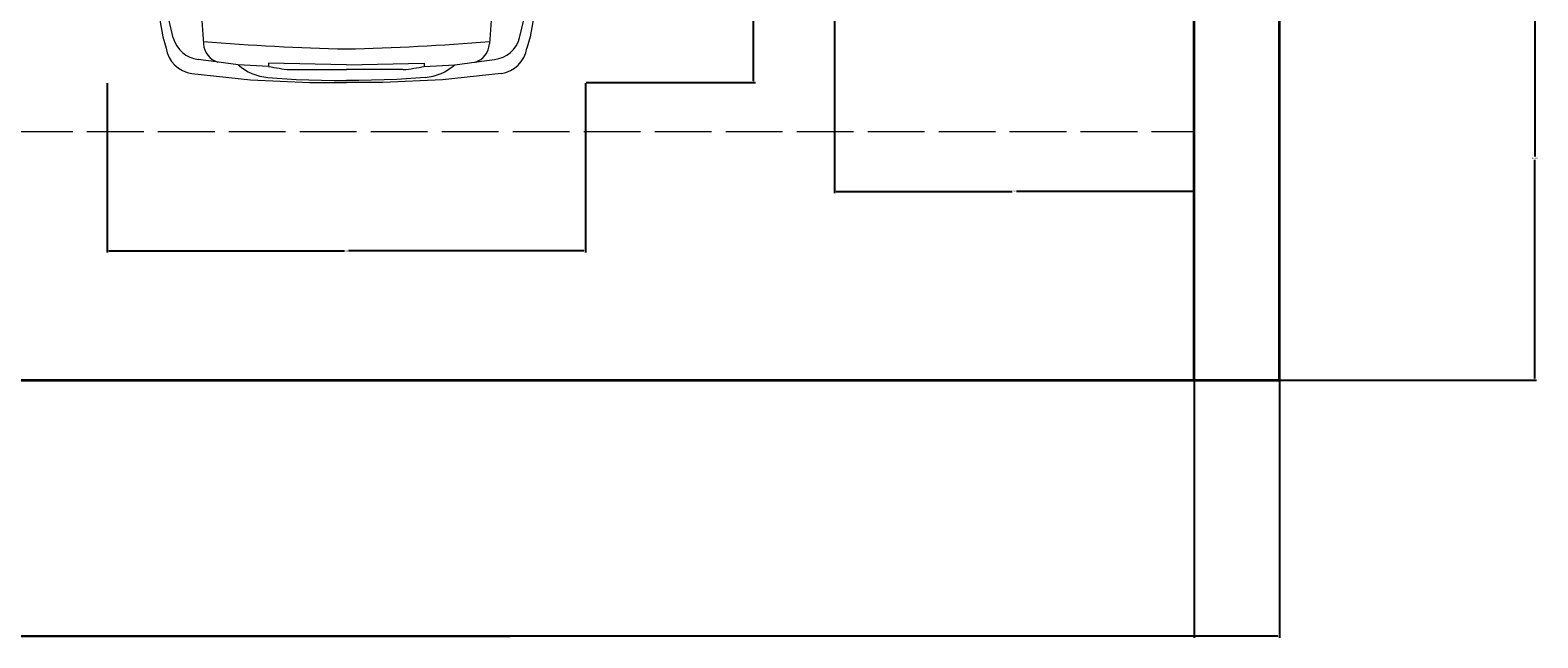
# Model space of a CAD drawing. Units: inches. Extents: x 2599 to 2953, y 557 to 1152.
# Tile 2 of 7: x 2794 to 2953, y 557 to 621. Entities that reach past the tile are written whole.
import ezdxf

# ---------------------------------------------------------------- set-up
doc = ezdxf.new("R2010")
doc.units = ezdxf.units.IN
doc.linetypes.add('ACAD_ISO02W100', pattern=[15, 12, -3])
for name, color, linetype, lineweight in [('0_Equip', 250, 'Continuous', 13), ('A-ANNO-DIMS', 2, 'Continuous', 18), ('A-WALL', 7, 'Continuous', 35), ('A-WALL-OVHD', 8, 'ACAD_ISO02W100', 18)]:
    doc.layers.add(name, color=color, linetype=linetype, lineweight=lineweight)
doc.styles.get("Standard").update_dxf_attribs({"font": 'arial.ttf'})
doc.dimstyles.get("Standard").update_dxf_attribs({"dimtxt": 0.18, "dimasz": 0.18, "dimexe": 0.18, "dimexo": 0.0625, "dimgap": 0.09, "dimtad": 0, "dimtih": 1, "dimtoh": 1, "dimdec": 4, "dimzin": 0, "dimdsep": 46, "dimtxsty": 'Standard', "dimcen": 0.09, "dimadec": 0, "dimazin": 0, "dimtfac": 1, "dimtdec": 4, "dimtofl": 0, "dimtmove": 0, "dimatfit": 3, "dimfxl": 1, "dimtolj": 1, "dimtzin": 0, "dimarcsym": 0})

# ---------------------------------------------------------------- blocks, each defined once
blk = doc.blocks.new('A$C4C7B54D1')
at = {"layer": '0_Equip', "ltscale": 0.1}
for p, q in [((-1.5486, -1.6107), (-1.5024, -1.8663)), ((0.0973, -1.6107), (0.0511, -1.8663)), ((-1.4584, -1.8701), (-1.4962, -1.7129)), ((-1.3433, -1.7188), (-1.3304, -1.8962)), ((-0.1081, -1.7188), (-0.1209, -1.8962)), ((0.0071, -1.8701), (0.0448, -1.7129)), ((-1.5024, -1.8663), (-1.4894, -1.914)), ((0.0511, -1.8663), (0.0381, -1.914)), ((-1.2767, -1.9721), (-1.3526, -1.9616)), ((-1.1845, -1.9838), (-1.2767, -1.9721)), ((-1.055, -1.9768), (-1.055, -1.9908)), ((-0.7257, -1.985), (-1.055, -1.9768)), ((-0.7257, -1.985), (-0.3964, -1.9768)), ((-0.3964, -1.9768), (-0.3964, -1.9908)), ((-0.2668, -1.9838), (-0.1746, -1.9721)), ((-0.1746, -1.9721), (-0.0987, -1.9616)), ((-1.3797, -2.0208), (-1.1314, -2.0483)), ((-1.055, -1.9908), (-1.1845, -1.9838)), ((-1.0585, -2.0375), (-0.9383, -2.0469)), ((-0.9663, -2.0048), (-0.7257, -2.0048)), ((-0.4851, -2.0048), (-0.7257, -2.0048)), ((-0.3929, -2.0375), (-0.5131, -2.0469)), ((-0.3964, -1.9908), (-0.2668, -1.9838)), ((-0.0716, -2.0208), (-0.3199, -2.0483)), ((-1.1314, -2.0483), (-0.8803, -2.0598)), ((-0.9383, -2.0469), (-0.7784, -2.0504)), ((-0.8803, -2.0598), (-0.7257, -2.0598)), ((-0.7784, -2.0504), (-0.7257, -2.0504)), ((-0.673, -2.0504), (-0.7257, -2.0504)), ((-0.5711, -2.0598), (-0.7257, -2.0598)), ((-0.5131, -2.0469), (-0.673, -2.0504)), ((-0.3199, -2.0483), (-0.5711, -2.0598))]:
    blk.add_line(p, q, dxfattribs=at)
for centre, radius, start, end in [((-1.3628, -1.8937), 0.1282, 189.09297, 262.41532), ((-1.3393, -1.8393), 0.123, 194.49857, 263.78362), ((-0.5134, 7.9307), 9.8503, 265.23745, 268.76503), ((-1.2452, -1.8915), 0.0853, 183.20552, 252.64053), ((-0.938, 7.9307), 9.8503, 271.23497, 274.76255), ((-0.2061, -1.8915), 0.0853, 287.35947, 356.79448), ((-0.1121, -1.8393), 0.123, 276.21638, 345.50143), ((-0.0885, -1.8937), 0.1282, 277.58468, 350.90703), ((-1.0413, -1.8225), 0.2157, 228.40601, 265.43909), ((-0.896, -1.272), 0.7362, 257.5275, 264.52088), ((-0.5554, -1.272), 0.7362, 275.47912, 282.4725), ((-0.41, -1.8225), 0.2157, 274.56091, 311.59399)]:
    blk.add_arc(centre, radius, start, end, dxfattribs=at)
blk = doc.blocks.new('*D19')
at = {"layer": 'A-ANNO-DIMS', "color": 0, "lineweight": -2, "transparency": 16777216}
for p, q in [((2852.68, 734.05), (2870.55, 734.05)), ((2870.37, 733.87), (2870.37, 675.09)), ((2870.37, 615.94), (2870.37, 674.72)), ((2852.68, 615.76), (2870.55, 615.76))]:
    blk.add_line(p, q, dxfattribs=at)
at = {"layer": 'A-ANNO-DIMS', "color": 0, "transparency": 16777216}
for points in [[(2870.34, 733.87), (2870.4, 733.87), (2870.37, 734.05)], [(2870.34, 615.94), (2870.4, 615.94), (2870.37, 615.76)]]:
    blk.add_solid(points, dxfattribs=at)
at = {"layer": 'Defpoints', "color": 0, "transparency": 16777216}
for p in [(2852.62, 734.05), (2870.37, 734.05), (2852.62, 615.76)]:
    blk.add_point(p, dxfattribs=at)
at = {"layer": 'A-ANNO-DIMS', "color": 0, "transparency": 16777216, "insert": (2870.37, 674.9), "char_height": 0.18, "attachment_point": 5}
blk.add_mtext('\\A1;CAR 118', dxfattribs=at)
blk = doc.blocks.new('*D20')
at = {"layer": 'A-ANNO-DIMS', "color": 0, "lineweight": -2, "transparency": 16777216}
for p, q in [((2802.07, 615.69), (2802.07, 597.83)), ((2852.62, 615.69), (2852.62, 597.83)), ((2802.25, 598.01), (2827.14, 598.01)), ((2852.44, 598.01), (2827.55, 598.01))]:
    blk.add_line(p, q, dxfattribs=at)
at = {"layer": 'A-ANNO-DIMS', "color": 0, "transparency": 16777216}
for points in [[(2802.25, 598.04), (2802.25, 597.98), (2802.07, 598.01)], [(2852.44, 598.04), (2852.44, 597.98), (2852.62, 598.01)]]:
    blk.add_solid(points, dxfattribs=at)
at = {"layer": 'Defpoints', "color": 0, "transparency": 16777216}
for p in [(2802.07, 615.76), (2852.62, 615.76), (2852.62, 598.01)]:
    blk.add_point(p, dxfattribs=at)
at = {"layer": 'A-ANNO-DIMS', "color": 0, "transparency": 16777216, "insert": (2827.35, 598.01), "char_height": 0.18, "attachment_point": 5}
blk.add_mtext('\\A1;51', dxfattribs=at)
blk = doc.blocks.new('*D21')
at = {"layer": 'A-ANNO-DIMS', "color": 0, "lineweight": -2, "transparency": 16777216}
for p, q in [((2625.92, 1124.28), (2625.92, 557.16)), ((2925.92, 584.28), (2925.92, 557.16)), ((2626.1, 557.34), (2775.63, 557.34)), ((2925.74, 557.34), (2776.21, 557.34))]:
    blk.add_line(p, q, dxfattribs=at)
at = {"layer": 'A-ANNO-DIMS', "color": 0, "transparency": 16777216}
for points in [[(2626.1, 557.37), (2626.1, 557.31), (2625.92, 557.34)], [(2925.74, 557.37), (2925.74, 557.31), (2925.92, 557.34)]]:
    blk.add_solid(points, dxfattribs=at)
at = {"layer": 'Defpoints', "color": 0, "transparency": 16777216}
for p in [(2625.92, 1124.34), (2925.92, 584.34), (2925.92, 557.34)]:
    blk.add_point(p, dxfattribs=at)
at = {"layer": 'A-ANNO-DIMS', "color": 0, "transparency": 16777216, "insert": (2775.92, 557.34), "char_height": 0.18, "attachment_point": 5}
blk.add_mtext('\\A1;300', dxfattribs=at)
blk = doc.blocks.new('*D36')
at = {"layer": 'A-ANNO-DIMS', "color": 0, "lineweight": -2, "transparency": 16777216}
for p, q in [((2772.92, 584.28), (2772.92, 557.16)), ((2916.92, 584.28), (2916.92, 557.16)), ((2773.1, 557.34), (2844.64, 557.34)), ((2916.74, 557.34), (2845.2, 557.34))]:
    blk.add_line(p, q, dxfattribs=at)
at = {"layer": 'A-ANNO-DIMS', "color": 0, "transparency": 16777216}
for points in [[(2773.1, 557.37), (2773.1, 557.31), (2772.92, 557.34)], [(2916.74, 557.37), (2916.74, 557.31), (2916.92, 557.34)]]:
    blk.add_solid(points, dxfattribs=at)
at = {"layer": 'Defpoints', "color": 0, "transparency": 16777216}
for p in [(2772.92, 584.34), (2916.92, 584.34), (2916.92, 557.34)]:
    blk.add_point(p, dxfattribs=at)
at = {"layer": 'A-ANNO-DIMS', "color": 0, "transparency": 16777216, "insert": (2844.92, 557.34), "char_height": 0.18, "attachment_point": 5}
blk.add_mtext('\\A1;144', dxfattribs=at)
blk = doc.blocks.new('*D40')
at = {"layer": 'A-ANNO-DIMS', "color": 0, "lineweight": -2, "transparency": 16777216}
for p, q in [((2878.92, 631.2), (2878.92, 604.08)), ((2916.92, 631.2), (2916.92, 604.08)), ((2879.1, 604.26), (2897.7, 604.26)), ((2916.74, 604.26), (2898.14, 604.26))]:
    blk.add_line(p, q, dxfattribs=at)
at = {"layer": 'A-ANNO-DIMS', "color": 0, "transparency": 16777216}
for points in [[(2879.1, 604.29), (2879.1, 604.23), (2878.92, 604.26)], [(2916.74, 604.29), (2916.74, 604.23), (2916.92, 604.26)]]:
    blk.add_solid(points, dxfattribs=at)
at = {"layer": 'Defpoints', "color": 0, "transparency": 16777216}
for p in [(2878.92, 631.26), (2916.92, 631.26), (2878.92, 604.26)]:
    blk.add_point(p, dxfattribs=at)
at = {"layer": 'A-ANNO-DIMS', "color": 0, "transparency": 16777216, "insert": (2897.92, 604.26), "char_height": 0.18, "attachment_point": 5}
blk.add_mtext('\\A1;38', dxfattribs=at)
blk = doc.blocks.new('*D42')
at = {"layer": 'A-ANNO-DIMS', "color": 0, "lineweight": -2, "transparency": 16777216}
for p, q in [((2916.98, 631.26), (2953.1, 631.26)), ((2952.92, 631.08), (2952.92, 607.98)), ((2952.92, 584.52), (2952.92, 607.62)), ((2916.98, 584.34), (2953.1, 584.34))]:
    blk.add_line(p, q, dxfattribs=at)
at = {"layer": 'A-ANNO-DIMS', "color": 0, "transparency": 16777216}
for points in [[(2952.89, 631.08), (2952.95, 631.08), (2952.92, 631.26)], [(2952.89, 584.52), (2952.95, 584.52), (2952.92, 584.34)]]:
    blk.add_solid(points, dxfattribs=at)
at = {"layer": 'Defpoints', "color": 0, "transparency": 16777216}
for p in [(2916.92, 631.26), (2952.92, 631.26), (2916.92, 584.34)]:
    blk.add_point(p, dxfattribs=at)
at = {"layer": 'A-ANNO-DIMS', "color": 0, "transparency": 16777216, "insert": (2952.92, 607.8), "char_height": 0.18, "attachment_point": 5}
blk.add_mtext('\\A1;46.92', dxfattribs=at)

msp = doc.modelspace()

# ---------------------------------------------------------------- linework, layer by layer
at = {"layer": 'A-WALL'}
for p, q in [((2925.9211, 584.3417), (2925.9211, 1124.3417)), ((2916.9211, 610.5917), (2916.9211, 761.3417)), ((2916.9211, 584.3417), (2916.9211, 610.5917)), ((2625.9211, 584.3417), (2925.9211, 584.3417))]:
    msp.add_line(p, q, dxfattribs=at)
at = {"layer": 'A-WALL-OVHD', "ltscale": 0.5}
msp.add_line((2694.9211, 610.5917), (2916.9211, 610.5917), dxfattribs=at)

# ---------------------------------------------------------------- block references
at = {"layer": '0_Equip', "xscale": 24.96754716209234, "yscale": 24.96754716209234, "zscale": 24.96754716209234}
msp.add_blockref('A$C4C7B54D1', (2845.4636, 667.1855), dxfattribs=at)

# ---------------------------------------------------------------- dimensions: what is measured, and where the dimension line sits
at = {"layer": 'A-ANNO-DIMS'}
for base, p1, p2, picture, middle in [((2925.9211, 557.3382), (2625.9211, 1124.3417), (2925.9211, 584.3417), '*D21', (2775.9211, 557.3382)), ((2852.6224, 598.0129), (2802.0685, 615.7567), (2852.6224, 615.7567), '*D20', (2827.3455, 598.0129)), ((2916.9211, 557.3382), (2772.9211, 584.3417), (2916.9211, 584.3417), '*D36', (2844.9211, 557.3382))]:
    dim = msp.add_linear_dim(base=base, p1=p1, p2=p2, dimstyle='Standard', override={"dimdec": 0, "dimlfac": 1, "dimrnd": 0, "dimzin": 0, "dimdsep": 46, "dimlunit": 2}, dxfattribs=at)
    dim.commit()
    dim.dimension.update_dxf_attribs({"geometry": picture, "text_midpoint": middle})
dim = msp.add_linear_dim(base=(2870.3661, 734.0485), p1=(2852.6224, 615.7567), p2=(2852.6224, 734.0485), angle=90, text='CAR <>', dimstyle='Standard', override={"dimdec": 0, "dimlfac": 1, "dimrnd": 0, "dimzin": 0, "dimdsep": 46, "dimlunit": 2}, dxfattribs=at)
dim.commit()
dim.dimension.update_dxf_attribs({"geometry": '*D19', "text_midpoint": (2870.3661, 674.9026)})
for base, p1, p2, angle, override, picture, middle in [((2878.9211, 604.2606), (2916.9211, 631.2641), (2878.9211, 631.2641), 180, {"dimdec": 0, "dimlfac": 1, "dimrnd": 0, "dimzin": 0, "dimdsep": 46, "dimlunit": 2}, '*D40', (2897.9211, 604.2606)), ((2952.9246, 631.2641), (2916.9211, 584.3417), (2916.9211, 631.2641), 90, {"dimdec": 2, "dimlfac": 1, "dimrnd": 0, "dimzin": 0, "dimdsep": 46, "dimlunit": 2}, '*D42', (2952.9246, 607.8029))]:
    dim = msp.add_linear_dim(base=base, p1=p1, p2=p2, angle=angle, dimstyle='Standard', override=override, dxfattribs=at)
    dim.commit()
    dim.dimension.update_dxf_attribs({"geometry": picture, "text_midpoint": middle})

doc.saveas('drawing.dxf')
